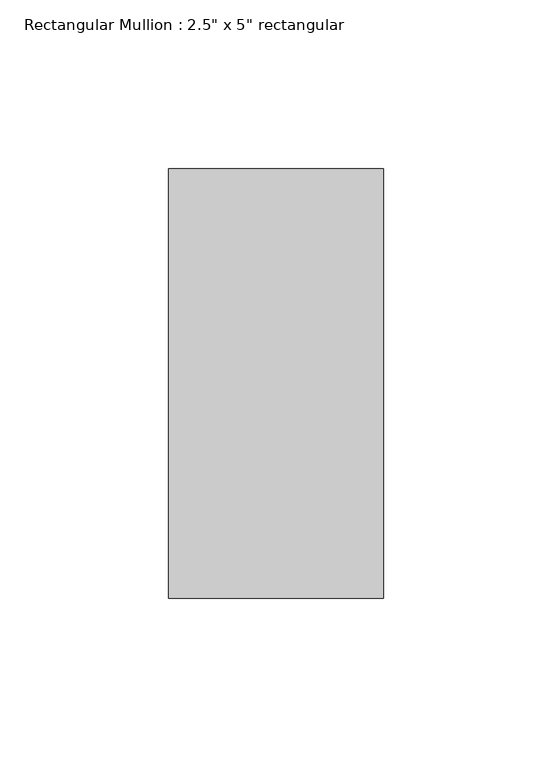
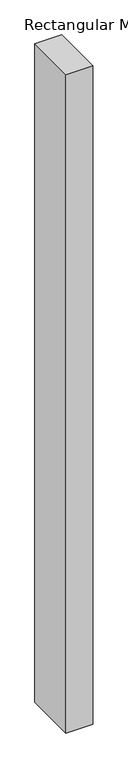
"""IFC4 building model written with IfcOpenShell, lengths in millimetres: member geometry."""

from ifc_helpers import new_model, si_unit, frame, origin, place, context, project, spatial, polyline, outline, extrude, source, transform, mapped, element, save


def member_2030dc42(model_context):
    return source(origin(), model_context, "Body", "SweptSolid", [
        extrude(outline(polyline([(0.0, 63.5), (0.0, -63.5), (-63.5, -63.5), (-63.5, 63.5), (0.0, 63.5)])), frame((0.0, 0.0, -1649.9537661), z_axis=(0.0, 0.0, 1.0), x_axis=(1.0, 0.0, 0.0)), (0.0, 0.0, 1.0), 1649.9537661),
    ])


if __name__ == "__main__":
    model = new_model("IFC4")
    model_context = context("Model", 3, world=origin())
    ifc_project = project(units=[si_unit("LENGTHUNIT", "METRE", prefix="MILLI")], contexts=[model_context])
    site = spatial("IfcSite", under=ifc_project)
    building = spatial("IfcBuilding", under=site)
    placement = place(None, origin())
    member_shape = member_2030dc42(model_context)
    element("IfcMember", 1, ObjectType="Rectangular Mullion : 2.5\" x 5\" rectangular", at=placement, inside=building, context=model_context, shape_type="MappedRepresentation", body=[
        mapped(member_shape, transform((0.0, 0.0, 0.0), x_axis=(1.0, 0.0, 0.0), y_axis=(0.0, 1.0, 0.0), z_axis=(0.0, 0.0, 1.0))),
    ])
    save(model, "model.ifc")

# Revit data of these elements
# Type "Rectangular Mullion : 2.5\" x 5\" rectangular"
#   built-in parameter 1007304 = 0.416667 (stored number, unit not read)
#   built-in parameter 1007301 = 0.104167 (stored number, unit not read)
#   built-in parameter 1007300 = 0.104167 (stored number, unit not read)
# Element 1 (IfcMember, "Rectangular Mullion : 2.5\" x 5\" rectangular")
#   Materials on its faces: "Aluminum"
# Materials
#   "Aluminum": class "Metal", colour RGB 247 247 247, transparency 0, Description = "Aluminum 6061", Cost = 0
